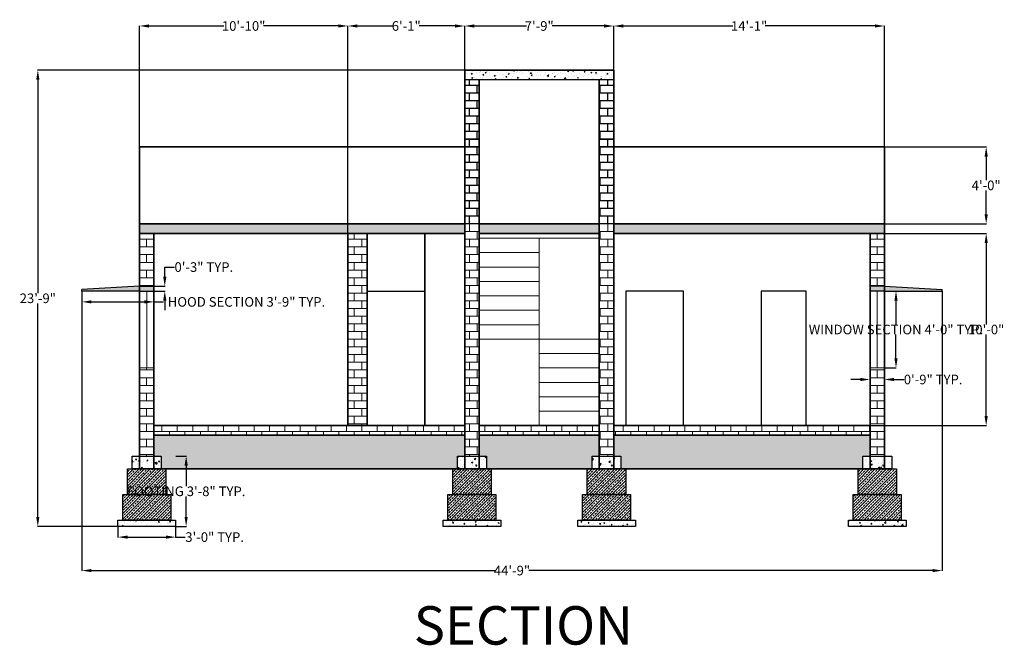
# Model space of a CAD drawing. Units: inches. Extents: x 1966 to 4198, y 2607 to 3884.
# Tile 3 of 8: x 2806 to 3420, y 2607 to 2998. Entities that reach past the tile are written whole.
import ezdxf

# ---------------------------------------------------------------- set-up
doc = ezdxf.new("R2010")
doc.units = ezdxf.units.IN
doc.header["$MEASUREMENT"] = 0
for name, color, linetype, lineweight in [('A-ANNO-TEXT', 4, 'Continuous', 25), ('A-FLOR-STRS', 7, 'Continuous', 18), ('A-GLAZ', 4, 'Continuous', 18), ('A-ROOF', 7, 'Continuous', 25), ('A-SECT', 7, 'Continuous', 35), ('A-SECT-PATT', 8, 'Continuous', 13), ('dimension', 90, 'Continuous', 18), ('door', 17, 'Continuous', 25), ('S-FNDN', 17, 'Continuous', 35)]:
    doc.layers.add(name, color=color, linetype=linetype, lineweight=lineweight)
doc.styles.get("Standard").update_dxf_attribs({"font": 'arial.ttf'})
doc.dimstyles.get("Standard").update_dxf_attribs({"dimtxt": 6, "dimasz": 6, "dimexe": 0.18, "dimexo": 0.0625, "dimgap": 0.09, "dimtad": 0, "dimtih": 1, "dimtoh": 1, "dimdec": 1, "dimzin": 0, "dimdsep": 46, "dimlunit": 3, "dimtxsty": 'Standard', "dimcen": 0.09, "dimadec": 0, "dimazin": 0, "dimtfac": 1, "dimtdec": 1, "dimtofl": 0, "dimtmove": 0, "dimatfit": 3, "dimfxl": 1, "dimtolj": 1, "dimtzin": 0, "dimarcsym": 0})
pattern_1 = [(50, (0, 0), (7.172602, -0.627521), [0.75, -8.25]), (355, (0, 0), (-1.387513, 7.521921), [0.6, -6.6]), (100.45144, (0.598, -0.052), (5.785088, 6.8944), [0.637402, -7.011421]), (46.1842, (0, 2), (10.672413, -1.655193), [1.125, -12.375]), (96.63564, (0.889, 1.862), (9.34662, 9.741186), [0.956103, -10.517138]), (351.18416, (0, 2), (9.34662, 9.741186), [0.9, -9.9]), (21, (1, 1.5), (5.9690705, -4.026189), [0.75, -8.25]), (326, (1, 1.5), (2.433153, 7.2515), [0.6, -6.6]), (71.45144, (1.4974, 1.1645), (8.402224, 3.225312), [0.637402, -7.011421]), (37.5, (0, 0), (0.1215986, 3.3289385), [0, -6.52, 0, -6.7, 0, -6.625]), (7.5, (0, 0), (2.6306954, 3.944117), [0, -3.82, 0, -6.37, 0, -2.525]), (327.5, (-2.23, 0), (5.3382244, -0.2255487), [0, -2.5, 0, -7.8, 0, -10.35]), (317.5, (-3.23, 0), (5.8318617, 1.00105), [0, -3.25, 0, -5.18, 0, -7.35])]

# ---------------------------------------------------------------- blocks, each defined once
blk = doc.blocks.new('FOUNDATION')
at = {"layer": 'door', "transparency": 33554577}
h = blk.add_hatch(dxfattribs=at)
h.set_pattern_fill('AR-CONC', color=256)
h.set_pattern_definition(pattern_1)
h.paths.add_polyline_path([(2817.43, 2606.1), (2817.43, 2602.1), (2853.43, 2602.1), (2853.43, 2606.1)])
h.paths.add_polyline_path([(2844.43, 2638.1), (2844.43, 2646.1), (2826.43, 2646.1), (2826.43, 2638.1)])
h = blk.add_hatch(dxfattribs=at)
h.set_pattern_fill('ANSI33', color=256, scale=10)
h.paths.add_polyline_path([(2847.43, 2622.1), (2847.43, 2638.1), (2823.43, 2638.1), (2823.43, 2622.1)])
h.paths.add_polyline_path([(2850.43, 2606.1), (2850.43, 2622.1), (2820.43, 2622.1), (2820.43, 2606.1)])
at = {"layer": 'door'}
for p, q in [((2826.43, 2646.1), (2844.43, 2646.1)), ((2826.43, 2638.1), (2826.43, 2646.1)), ((2844.43, 2646.1), (2844.43, 2638.1)), ((2823.43, 2638.1), (2847.43, 2638.1)), ((2823.43, 2622.1), (2823.43, 2638.1)), ((2844.43, 2638.1), (2826.43, 2638.1)), ((2847.43, 2638.1), (2847.43, 2622.1)), ((2820.43, 2622.1), (2850.43, 2622.1)), ((2820.43, 2606.1), (2820.43, 2622.1)), ((2847.43, 2622.1), (2823.43, 2622.1)), ((2850.43, 2622.1), (2850.43, 2606.1)), ((2817.43, 2606.1), (2853.43, 2606.1)), ((2817.43, 2602.1), (2817.43, 2606.1)), ((2850.43, 2606.1), (2820.43, 2606.1)), ((2853.43, 2606.1), (2853.43, 2602.1)), ((2853.43, 2602.1), (2817.43, 2602.1))]:
    blk.add_line(p, q, dxfattribs=at)
blk = doc.blocks.new('WINDOW-SECTION')
blk.add_line((4.5, 0), (4.5, 48))
blk.add_lwpolyline([(0, 48), (9, 48), (9, 0), (0, 0)], close=True)
blk = doc.blocks.new('WINDOW-HOOD-SECTION')
for p, q in [((36, 3), (0, 1)), ((0, 0), (0, 1)), ((36, 0), (0, 0)), ((36, 3), (45, 3)), ((36, 0), (45, 0))]:
    blk.add_line(p, q)
blk = doc.blocks.new('*D45')
at = {"layer": 'Defpoints', "color": 0, "transparency": 16777216}
for p in [(2902.94, 2725.47), (2909.54, 2725.47), (2902.94, 2681.47)]:
    blk.add_point(p, dxfattribs=at)
at = {"layer": 'dimension', "color": 0, "lineweight": -2, "transparency": 16777216}
for p, q in [((2903, 2725.47), (2909.72, 2725.47)), ((2909.54, 2719.47), (2909.54, 2706.66)), ((2909.54, 2687.47), (2909.54, 2700.27)), ((2903, 2681.47), (2909.72, 2681.47))]:
    blk.add_line(p, q, dxfattribs=at)
at = {"layer": 'dimension', "color": 0, "transparency": 16777216}
for points in [[(2908.54, 2719.47), (2910.54, 2719.47), (2909.54, 2725.47)], [(2908.54, 2687.47), (2910.54, 2687.47), (2909.54, 2681.47)]]:
    blk.add_solid(points, dxfattribs=at)
at = {"layer": 'dimension', "color": 0, "transparency": 16777216, "insert": (2909.54, 2703.47), "char_height": 6, "attachment_point": 5}
blk.add_mtext('\\A1;FOOTING 3\'-8" TYP.', dxfattribs=at)
blk = doc.blocks.new('*D46')
at = {"layer": 'Defpoints', "color": 0, "transparency": 16777216}
for p in [(2866.94, 2681.47), (2902.94, 2681.47), (2902.94, 2674.87)]:
    blk.add_point(p, dxfattribs=at)
at = {"layer": 'dimension', "color": 0, "lineweight": -2, "transparency": 16777216}
for p, q in [((2866.94, 2681.4), (2866.94, 2674.69)), ((2902.94, 2681.4), (2902.94, 2674.69)), ((2872.94, 2674.87), (2896.94, 2674.87)), ((2902.94, 2674.87), (2908.94, 2674.87))]:
    blk.add_line(p, q, dxfattribs=at)
at = {"layer": 'dimension', "color": 0, "transparency": 16777216}
for points in [[(2872.94, 2675.87), (2872.94, 2673.87), (2866.94, 2674.87)], [(2896.94, 2675.87), (2896.94, 2673.87), (2902.94, 2674.87)]]:
    blk.add_solid(points, dxfattribs=at)
at = {"layer": 'dimension', "color": 0, "transparency": 16777216, "insert": (2927.32, 2674.87), "char_height": 6, "attachment_point": 5}
blk.add_mtext('\\A1;3\'-0" TYP.', dxfattribs=at)
blk = doc.blocks.new('*D71')
at = {"layer": 'Defpoints', "color": 0, "transparency": 16777216}
for p in [(2844.44, 2828.47), (2889.44, 2828.47), (2889.44, 2821.72)]:
    blk.add_point(p, dxfattribs=at)
at = {"layer": 'dimension', "color": 0, "lineweight": -2, "transparency": 16777216}
for p, q in [((2844.44, 2828.4), (2844.44, 2821.54)), ((2889.44, 2828.4), (2889.44, 2821.54)), ((2850.44, 2821.72), (2883.44, 2821.72)), ((2889.44, 2821.72), (2895.44, 2821.72))]:
    blk.add_line(p, q, dxfattribs=at)
at = {"layer": 'dimension', "color": 0, "transparency": 16777216}
for points in [[(2850.44, 2822.72), (2850.44, 2820.72), (2844.44, 2821.72)], [(2883.44, 2822.72), (2883.44, 2820.72), (2889.44, 2821.72)]]:
    blk.add_solid(points, dxfattribs=at)
at = {"layer": 'dimension', "color": 0, "transparency": 16777216, "insert": (2947.19, 2821.72), "char_height": 6, "attachment_point": 5}
blk.add_mtext('\\A1;HOOD SECTION 3\'-9" TYP.', dxfattribs=at)
blk = doc.blocks.new('*D72')
at = {"layer": 'Defpoints', "color": 0, "transparency": 16777216}
for p in [(2889.44, 2831.47), (2889.44, 2828.47), (2896.19, 2831.47)]:
    blk.add_point(p, dxfattribs=at)
at = {"layer": 'dimension', "color": 0, "lineweight": -2, "transparency": 16777216}
for p, q in [((2896.19, 2837.47), (2896.19, 2843.47)), ((2896.19, 2843.47), (2902.19, 2843.47)), ((2889.5, 2831.47), (2896.37, 2831.47)), ((2889.5, 2828.47), (2896.37, 2828.47)), ((2896.19, 2822.47), (2896.19, 2816.47))]:
    blk.add_line(p, q, dxfattribs=at)
at = {"layer": 'dimension', "color": 0, "transparency": 16777216}
for points in [[(2895.19, 2837.47), (2897.19, 2837.47), (2896.19, 2831.47)], [(2895.19, 2822.47), (2897.19, 2822.47), (2896.19, 2828.47)]]:
    blk.add_solid(points, dxfattribs=at)
at = {"layer": 'dimension', "color": 0, "transparency": 16777216, "insert": (2920.57, 2843.47), "char_height": 6, "attachment_point": 5}
blk.add_mtext('\\A1;0\'-3" TYP.', dxfattribs=at)
blk = doc.blocks.new('*D73')
at = {"layer": 'Defpoints', "color": 0, "transparency": 16777216}
for p in [(3345.44, 2828.47), (3352.64, 2828.47), (3345.44, 2780.47)]:
    blk.add_point(p, dxfattribs=at)
at = {"layer": 'dimension', "color": 0, "lineweight": -2, "transparency": 16777216}
for p, q in [((3345.5, 2828.47), (3352.82, 2828.47)), ((3352.64, 2822.47), (3352.64, 2807.66)), ((3352.64, 2786.47), (3352.64, 2801.27)), ((3345.5, 2780.47), (3352.82, 2780.47))]:
    blk.add_line(p, q, dxfattribs=at)
at = {"layer": 'dimension', "color": 0, "transparency": 16777216}
for points in [[(3351.64, 2822.47), (3353.64, 2822.47), (3352.64, 2828.47)], [(3351.64, 2786.47), (3353.64, 2786.47), (3352.64, 2780.47)]]:
    blk.add_solid(points, dxfattribs=at)
at = {"layer": 'dimension', "color": 0, "transparency": 16777216, "insert": (3352.64, 2804.47), "char_height": 6, "attachment_point": 5}
blk.add_mtext('\\A1;WINDOW SECTION 4\'-0" TYP.', dxfattribs=at)
blk = doc.blocks.new('*D74')
at = {"layer": 'Defpoints', "color": 0, "transparency": 16777216}
for p in [(3336.44, 2780.47), (3345.44, 2780.47), (3345.44, 2773.27)]:
    blk.add_point(p, dxfattribs=at)
at = {"layer": 'dimension', "color": 0, "lineweight": -2, "transparency": 16777216}
for p, q in [((3336.44, 2780.4), (3336.44, 2773.09)), ((3345.44, 2780.4), (3345.44, 2773.09)), ((3330.44, 2773.27), (3324.44, 2773.27)), ((3351.44, 2773.27), (3357.44, 2773.27))]:
    blk.add_line(p, q, dxfattribs=at)
at = {"layer": 'dimension', "color": 0, "transparency": 16777216}
for points in [[(3330.44, 2774.27), (3330.44, 2772.27), (3336.44, 2773.27)], [(3351.44, 2774.27), (3351.44, 2772.27), (3345.44, 2773.27)]]:
    blk.add_solid(points, dxfattribs=at)
at = {"layer": 'dimension', "color": 0, "transparency": 16777216, "insert": (3375.82, 2773.27), "char_height": 6, "attachment_point": 5}
blk.add_mtext('\\A1;0\'-9" TYP.', dxfattribs=at)
blk = doc.blocks.new('*D112')
at = {"layer": 'Defpoints', "color": 0, "transparency": 16777216}
for p in [(2844.44, 2828.47), (3381.44, 2828.47), (3381.44, 2653.97)]:
    blk.add_point(p, dxfattribs=at)
at = {"layer": 'dimension', "color": 0, "lineweight": -2, "transparency": 16777216}
for p, q in [((2844.44, 2828.4), (2844.44, 2653.79)), ((3381.44, 2828.4), (3381.44, 2653.79)), ((2850.44, 2653.97), (3102.42, 2653.97)), ((3375.44, 2653.97), (3123.46, 2653.97))]:
    blk.add_line(p, q, dxfattribs=at)
at = {"layer": 'dimension', "color": 0, "transparency": 16777216}
for points in [[(2850.44, 2654.97), (2850.44, 2652.97), (2844.44, 2653.97)], [(3375.44, 2654.97), (3375.44, 2652.97), (3381.44, 2653.97)]]:
    blk.add_solid(points, dxfattribs=at)
at = {"layer": 'dimension', "color": 0, "transparency": 16777216, "insert": (3112.94, 2653.97), "char_height": 6, "attachment_point": 5}
blk.add_mtext('\\A1;44\'-9"', dxfattribs=at)
blk = doc.blocks.new('*D113')
at = {"layer": 'Defpoints', "color": 0, "transparency": 16777216}
for p in [(2816.94, 2966.47), (3083.44, 2966.47), (2866.94, 2681.47)]:
    blk.add_point(p, dxfattribs=at)
at = {"layer": 'dimension', "color": 0, "lineweight": -2, "transparency": 16777216}
for p, q in [((3083.38, 2966.47), (2816.76, 2966.47)), ((2816.94, 2960.47), (2816.94, 2827.12)), ((2816.94, 2687.47), (2816.94, 2820.81)), ((2866.88, 2681.47), (2816.76, 2681.47))]:
    blk.add_line(p, q, dxfattribs=at)
at = {"layer": 'dimension', "color": 0, "transparency": 16777216}
for points in [[(2815.94, 2960.47), (2817.94, 2960.47), (2816.94, 2966.47)], [(2815.94, 2687.47), (2817.94, 2687.47), (2816.94, 2681.47)]]:
    blk.add_solid(points, dxfattribs=at)
at = {"layer": 'dimension', "color": 0, "transparency": 16777216, "insert": (2816.94, 2823.97), "char_height": 6, "attachment_point": 5}
blk.add_mtext('\\A1;23\'-9"', dxfattribs=at)
blk = doc.blocks.new('*D114')
at = {"layer": 'Defpoints', "color": 0, "transparency": 16777216}
for p in [(3336.44, 2864.47), (3408.94, 2864.47), (3336.44, 2744.47)]:
    blk.add_point(p, dxfattribs=at)
at = {"layer": 'dimension', "color": 0, "lineweight": -2, "transparency": 16777216}
for p, q in [((3336.5, 2864.47), (3409.12, 2864.47)), ((3408.94, 2858.47), (3408.94, 2807.62)), ((3408.94, 2750.47), (3408.94, 2801.31)), ((3336.5, 2744.47), (3409.12, 2744.47))]:
    blk.add_line(p, q, dxfattribs=at)
at = {"layer": 'dimension', "color": 0, "transparency": 16777216}
for points in [[(3407.94, 2858.47), (3409.94, 2858.47), (3408.94, 2864.47)], [(3407.94, 2750.47), (3409.94, 2750.47), (3408.94, 2744.47)]]:
    blk.add_solid(points, dxfattribs=at)
at = {"layer": 'dimension', "color": 0, "transparency": 16777216, "insert": (3408.94, 2804.47), "char_height": 6, "attachment_point": 5}
blk.add_mtext('\\A1;10\'-0"', dxfattribs=at)
blk = doc.blocks.new('*D115')
at = {"layer": 'Defpoints', "color": 0, "transparency": 16777216}
for p in [(3010.44, 2993.97), (2880.44, 2864.47), (3010.44, 2864.47)]:
    blk.add_point(p, dxfattribs=at)
at = {"layer": 'dimension', "color": 0, "lineweight": -2, "transparency": 16777216}
for p, q in [((2880.44, 2864.53), (2880.44, 2994.15)), ((2886.44, 2993.97), (2933, 2993.97)), ((3004.44, 2993.97), (2957.88, 2993.97)), ((3010.44, 2864.53), (3010.44, 2994.15))]:
    blk.add_line(p, q, dxfattribs=at)
at = {"layer": 'dimension', "color": 0, "transparency": 16777216}
for points in [[(2886.44, 2994.97), (2886.44, 2992.97), (2880.44, 2993.97)], [(3004.44, 2994.97), (3004.44, 2992.97), (3010.44, 2993.97)]]:
    blk.add_solid(points, dxfattribs=at)
at = {"layer": 'dimension', "color": 0, "transparency": 16777216, "insert": (2945.44, 2993.97), "char_height": 6, "attachment_point": 5}
blk.add_mtext('\\A1;10\'-10"', dxfattribs=at)
blk = doc.blocks.new('*D116')
at = {"layer": 'Defpoints', "color": 0, "transparency": 16777216}
for p in [(3083.44, 2993.97), (3083.44, 2918.47), (3010.44, 2864.47)]:
    blk.add_point(p, dxfattribs=at)
at = {"layer": 'dimension', "color": 0, "lineweight": -2, "transparency": 16777216}
for p, q in [((3010.44, 2864.53), (3010.44, 2994.15)), ((3016.44, 2993.97), (3038.86, 2993.97)), ((3077.44, 2993.97), (3055.02, 2993.97)), ((3083.44, 2918.53), (3083.44, 2994.15))]:
    blk.add_line(p, q, dxfattribs=at)
at = {"layer": 'dimension', "color": 0, "transparency": 16777216}
for points in [[(3016.44, 2994.97), (3016.44, 2992.97), (3010.44, 2993.97)], [(3077.44, 2994.97), (3077.44, 2992.97), (3083.44, 2993.97)]]:
    blk.add_solid(points, dxfattribs=at)
at = {"layer": 'dimension', "color": 0, "transparency": 16777216, "insert": (3046.94, 2993.97), "char_height": 6, "attachment_point": 5}
blk.add_mtext('\\A1;6\'-1"', dxfattribs=at)
blk = doc.blocks.new('*D117')
at = {"layer": 'Defpoints', "color": 0, "transparency": 16777216}
for p in [(3176.44, 2993.97), (3083.44, 2966.47), (3176.44, 2966.42)]:
    blk.add_point(p, dxfattribs=at)
at = {"layer": 'dimension', "color": 0, "lineweight": -2, "transparency": 16777216}
for p, q in [((3083.44, 2966.53), (3083.44, 2994.15)), ((3089.44, 2993.97), (3121.9, 2993.97)), ((3170.44, 2993.97), (3137.98, 2993.97)), ((3176.44, 2966.49), (3176.44, 2994.15))]:
    blk.add_line(p, q, dxfattribs=at)
at = {"layer": 'dimension', "color": 0, "transparency": 16777216}
for points in [[(3089.44, 2994.97), (3089.44, 2992.97), (3083.44, 2993.97)], [(3170.44, 2994.97), (3170.44, 2992.97), (3176.44, 2993.97)]]:
    blk.add_solid(points, dxfattribs=at)
at = {"layer": 'dimension', "color": 0, "transparency": 16777216, "insert": (3129.94, 2993.97), "char_height": 6, "attachment_point": 5}
blk.add_mtext('\\A1;7\'-9"', dxfattribs=at)
blk = doc.blocks.new('*D118')
at = {"layer": 'Defpoints', "color": 0, "transparency": 16777216}
for p in [(3345.44, 2993.97), (3176.44, 2918.47), (3345.44, 2918.47)]:
    blk.add_point(p, dxfattribs=at)
at = {"layer": 'dimension', "color": 0, "lineweight": -2, "transparency": 16777216}
for p, q in [((3176.44, 2918.53), (3176.44, 2994.15)), ((3182.44, 2993.97), (3250.83, 2993.97)), ((3339.44, 2993.97), (3271.05, 2993.97)), ((3345.44, 2918.53), (3345.44, 2994.15))]:
    blk.add_line(p, q, dxfattribs=at)
at = {"layer": 'dimension', "color": 0, "transparency": 16777216}
for points in [[(3182.44, 2994.97), (3182.44, 2992.97), (3176.44, 2993.97)], [(3339.44, 2994.97), (3339.44, 2992.97), (3345.44, 2993.97)]]:
    blk.add_solid(points, dxfattribs=at)
at = {"layer": 'dimension', "color": 0, "transparency": 16777216, "insert": (3260.94, 2993.97), "char_height": 6, "attachment_point": 5}
blk.add_mtext('\\A1;14\'-1"', dxfattribs=at)
blk = doc.blocks.new('*D119')
at = {"layer": 'Defpoints', "color": 0, "transparency": 16777216}
for p in [(3345.44, 2918.47), (3408.94, 2918.47), (3345.44, 2870.47)]:
    blk.add_point(p, dxfattribs=at)
at = {"layer": 'dimension', "color": 0, "lineweight": -2, "transparency": 16777216}
for p, q in [((3345.5, 2918.47), (3409.12, 2918.47)), ((3408.94, 2912.47), (3408.94, 2897.62)), ((3408.94, 2876.47), (3408.94, 2891.31)), ((3345.5, 2870.47), (3409.12, 2870.47))]:
    blk.add_line(p, q, dxfattribs=at)
at = {"layer": 'dimension', "color": 0, "transparency": 16777216}
for points in [[(3407.94, 2912.47), (3409.94, 2912.47), (3408.94, 2918.47)], [(3407.94, 2876.47), (3409.94, 2876.47), (3408.94, 2870.47)]]:
    blk.add_solid(points, dxfattribs=at)
at = {"layer": 'dimension', "color": 0, "transparency": 16777216, "insert": (3408.94, 2894.47), "char_height": 6, "attachment_point": 5}
blk.add_mtext('\\A1;4\'-0"', dxfattribs=at)

msp = doc.modelspace()

# ---------------------------------------------------------------- hatches: boundary and pattern name
at = {"layer": 'A-SECT-PATT', "transparency": 33554577}
h = msp.add_hatch(dxfattribs=at)
h.set_pattern_fill('AR-CONC', color=256)
h.set_pattern_definition(pattern_1)
h.paths.add_polyline_path([(3176.44, 2966.42), (3083.44, 2966.47), (3083.44, 2960.47), (3176.44, 2960.42)])
h = msp.add_hatch(dxfattribs=at)
h.set_pattern_fill('AR-B816C', color=256, scale=0.6)
h.paths.add_polyline_path([(3092.44, 2960.46), (3083.44, 2960.47), (3083.44, 2870.47), (3092.44, 2870.47)])
h.paths.add_polyline_path([(3176.44, 2960.42), (3167.44, 2960.43), (3167.44, 2870.47), (3176.44, 2870.47)])
h = msp.add_hatch(dxfattribs=at)
h.set_pattern_fill('AR-B816', color=256, scale=0.6)
h.paths.add_polyline_path([(2889.44, 2780.47), (2880.44, 2780.47), (2880.44, 2725.47), (2889.44, 2725.47)])
h.paths.add_polyline_path([(2889.44, 2864.47), (2880.44, 2864.47), (2880.44, 2831.47), (2889.44, 2831.47)])
h.paths.add_polyline_path([(3022.44, 2864.47), (3010.44, 2864.47), (3010.44, 2744.47), (3022.44, 2744.47)])
h.paths.add_polyline_path([(3092.44, 2870.44), (3083.44, 2870.44), (3083.44, 2725.47), (3092.44, 2725.47)])
h.paths.add_polyline_path([(3176.44, 2870.73), (3167.44, 2870.73), (3167.44, 2725.47), (3176.44, 2725.47)])
h.paths.add_polyline_path([(3345.44, 2864.47), (3336.44, 2864.47), (3336.44, 2831.47), (3345.44, 2831.47)])
h.paths.add_polyline_path([(3345.44, 2780.47), (3336.44, 2780.47), (3336.44, 2725.47), (3345.44, 2725.47)])
h.paths.add_polyline_path([(3083.44, 2744.47), (3058.44, 2744.47), (2889.44, 2744.47), (2889.44, 2738.47), (3083.44, 2738.47)])
h.paths.add_polyline_path([(3129.94, 2744.47), (3092.44, 2744.47), (3092.44, 2738.47), (3129.94, 2738.47)])
h.paths.add_polyline_path([(3167.44, 2744.47), (3129.94, 2744.47), (3129.94, 2738.47), (3167.44, 2738.47)])
h.paths.add_polyline_path([(3336.44, 2744.47), (3176.44, 2744.47), (3176.44, 2738.47), (3336.44, 2738.47)])
h = msp.add_hatch(dxfattribs=at)
h.set_pattern_fill('AR-CONC', color=256)
h.set_pattern_definition(pattern_1)
h.paths.add_polyline_path([(3083.44, 2864.47), (3083.44, 2870.47), (2880.44, 2870.47), (2880.44, 2864.47)])
h.paths.add_polyline_path([(3167.44, 2864.47), (3167.44, 2870.47), (3092.44, 2870.47), (3092.44, 2864.47)])
h.paths.add_polyline_path([(3176.44, 2870.47), (3176.44, 2864.47), (3345.44, 2864.47), (3345.44, 2870.47)])
h = msp.add_hatch(dxfattribs=at)
h.set_pattern_fill('AR-CONC', color=256)
h.set_pattern_definition(pattern_1)
h.paths.add_polyline_path([(2880.44, 2831.47), (2844.44, 2829.47), (2844.44, 2828.47), (2880.44, 2828.47)])
h.paths.add_polyline_path([(2889.44, 2831.47), (2880.44, 2831.47), (2880.44, 2828.47), (2889.44, 2828.47)])
h.paths.add_polyline_path([(3345.44, 2831.47), (3336.44, 2831.47), (3336.44, 2828.47), (3345.44, 2828.47)])
h.paths.add_polyline_path([(3345.44, 2831.47), (3345.44, 2828.47), (3381.44, 2828.47), (3381.44, 2829.47)])
h = msp.add_hatch(dxfattribs=at)
h.set_pattern_fill('AR-CONC', color=256)
h.set_pattern_definition(pattern_1)
h.paths.add_polyline_path([(3078.94, 2725.47), (3083.44, 2725.47), (3083.44, 2738.47), (2889.44, 2738.47), (2889.44, 2725.47), (2893.94, 2725.47), (2893.94, 2717.47), (2896.94, 2717.47), (3078.94, 2717.47)])
h.paths.add_polyline_path([(3167.44, 2738.47), (3092.44, 2738.47), (3092.44, 2725.47), (3096.94, 2725.47), (3096.94, 2717.47), (3099.94, 2717.47), (3162.94, 2717.47), (3162.94, 2725.47), (3167.44, 2725.47)])
h.paths.add_polyline_path([(3336.44, 2738.47), (3176.44, 2738.47), (3176.44, 2725.47), (3180.94, 2725.47), (3180.94, 2717.47), (3183.94, 2717.47), (3331.94, 2717.47), (3331.94, 2725.47), (3336.44, 2725.47)])

# ---------------------------------------------------------------- linework, layer by layer
at = {"layer": 'A-FLOR-STRS'}
for p, q in [((3092.44, 2861.47), (3167.44, 2861.47)), ((3129.94, 2744.47), (3129.94, 2861.47)), ((3092.44, 2852.47), (3129.94, 2852.47)), ((3092.44, 2843.47), (3129.94, 2843.47)), ((3092.44, 2834.47), (3129.94, 2834.47)), ((3092.44, 2825.47), (3129.94, 2825.47)), ((3092.44, 2816.47), (3129.94, 2816.47)), ((3092.44, 2807.47), (3129.94, 2807.47)), ((3092.44, 2798.47), (3167.44, 2798.47)), ((3129.94, 2789.47), (3167.44, 2789.47)), ((3129.94, 2780.47), (3167.44, 2780.47)), ((3129.94, 2771.47), (3167.44, 2771.47)), ((3129.94, 2762.47), (3167.44, 2762.47)), ((3129.94, 2753.47), (3167.44, 2753.47))]:
    msp.add_line(p, q, dxfattribs=at)
at = {"layer": 'A-SECT'}
for p, q in [((3083.44, 2966.47), (3176.44, 2966.42)), ((3083.44, 2966.47), (3083.44, 2960.47)), ((3176.44, 2966.42), (3176.44, 2960.42)), ((3083.44, 2864.47), (3083.44, 2960.47)), ((3083.44, 2960.47), (3176.44, 2960.42)), ((3092.44, 2864.47), (3092.44, 2960.47)), ((3167.44, 2960.42), (3167.44, 2864.47)), ((3176.44, 2960.42), (3176.44, 2864.47)), ((2880.44, 2918.47), (2880.44, 2717.47)), ((2880.44, 2918.47), (3083.44, 2918.47)), ((3176.44, 2918.47), (3345.44, 2918.47)), ((3345.44, 2918.47), (3345.44, 2717.47)), ((2880.44, 2870.47), (3083.44, 2870.47)), ((3092.44, 2870.47), (3167.44, 2870.47)), ((3176.44, 2870.47), (3345.44, 2870.47)), ((2880.44, 2864.47), (3083.44, 2864.47)), ((2889.44, 2864.47), (2889.44, 2717.47)), ((3010.44, 2864.47), (3010.44, 2744.47)), ((3022.44, 2744.47), (3022.44, 2864.47)), ((3058.44, 2744.47), (3058.44, 2864.47)), ((3083.44, 2864.47), (3083.44, 2717.47)), ((3092.44, 2864.47), (3092.44, 2717.47)), ((3092.44, 2864.47), (3167.44, 2864.47)), ((3167.44, 2864.47), (3167.44, 2717.47)), ((3176.44, 2864.47), (3176.44, 2717.47)), ((3176.44, 2864.47), (3345.44, 2864.47)), ((3336.44, 2864.47), (3336.44, 2717.47)), ((2889.44, 2744.47), (3083.44, 2744.47)), ((3092.44, 2744.47), (3167.44, 2744.47)), ((3176.44, 2744.47), (3336.44, 2744.47)), ((2889.44, 2738.47), (3083.44, 2738.47)), ((3092.44, 2738.47), (3167.44, 2738.47)), ((3176.44, 2738.47), (3336.44, 2738.47)), ((2880.44, 2717.47), (3345.44, 2717.47))]:
    msp.add_line(p, q, dxfattribs=at)
at = {"layer": 'door'}
for points in [[(3022.44, 2828.47), (3058.44, 2828.47), (3058.44, 2744.47), (3022.44, 2744.47)], [(3183.92, 2744.47), (3219.92, 2744.47), (3219.92, 2828.47), (3183.92, 2828.47)], [(3268.55, 2744.47), (3296.55, 2744.47), (3296.55, 2828.47), (3268.55, 2828.47)]]:
    msp.add_lwpolyline(points, close=True, dxfattribs=at)
at = {"layer": 'S-FNDN'}
for p, q in [((2880.44, 2717.47), (2889.44, 2717.47)), ((3083.44, 2717.47), (3092.44, 2717.47)), ((3167.44, 2717.47), (3176.44, 2717.47)), ((3336.44, 2717.47), (3345.44, 2717.47))]:
    msp.add_line(p, q, dxfattribs=at)

# ---------------------------------------------------------------- block references
at = {"layer": 'A-GLAZ'}
for p in [(2880.44, 2780.47), (3336.44, 2780.47)]:
    msp.add_blockref('WINDOW-SECTION', p, dxfattribs=at)
at = {"layer": 'A-ROOF'}
msp.add_blockref('WINDOW-HOOD-SECTION', (2844.44, 2828.47), dxfattribs=at)
at = {"layer": 'A-ROOF', "extrusion": (0, 0, -1), "zscale": -1}
msp.add_blockref('WINDOW-HOOD-SECTION', (-3381.44, 2828.47), dxfattribs=at)
at = {"layer": 'S-FNDN'}
for p in [(49.51, 79.37), (252.51, 79.37), (336.51, 79.37), (505.51, 79.37)]:
    msp.add_blockref('FOUNDATION', p, dxfattribs=at)

# ---------------------------------------------------------------- texts
at = {"layer": 'A-ANNO-TEXT', "insert": (3120.06, 2631.74), "char_height": 24, "attachment_point": 2}
msp.add_mtext_dynamic_manual_height_columns('SECTION', width=89.9452, gutter_width=1, heights=[0], dxfattribs=at)

# ---------------------------------------------------------------- dimensions: what is measured, and where the dimension line sits
at = {"layer": 'dimension'}
for base, p1, p2, picture, middle in [((3010.44, 2993.97), (2880.44, 2864.47), (3010.44, 2864.47), '*D115', (2945.44, 2993.97)), ((3083.44, 2993.97), (3010.44, 2864.47), (3083.44, 2918.47), '*D116', (3046.94, 2993.97)), ((3176.44, 2993.97), (3083.44, 2966.47), (3176.44, 2966.42), '*D117', (3129.94, 2993.97)), ((3345.44, 2993.97), (3176.44, 2918.47), (3345.44, 2918.47), '*D118', (3260.94, 2993.97)), ((3381.44, 2653.97), (2844.44, 2828.47), (3381.44, 2828.47), '*D112', (3112.94, 2653.97))]:
    dim = msp.add_linear_dim(base=base, p1=p1, p2=p2, dimstyle='Standard', override={"dimdec": 1, "dimlfac": 1, "dimrnd": 0, "dimzin": 1, "dimdsep": 46, "dimlunit": 4, "dimfrac": 2}, dxfattribs=at)
    dim.commit()
    dim.dimension.update_dxf_attribs({"geometry": picture, "text_midpoint": middle})
for base, p1, p2, picture, middle in [((2816.94, 2966.47), (2866.94, 2681.47), (3083.44, 2966.47), '*D113', (2816.94, 2823.97)), ((3408.94, 2918.47), (3345.44, 2870.47), (3345.44, 2918.47), '*D119', (3408.94, 2894.47)), ((3408.94, 2864.47), (3336.44, 2744.47), (3336.44, 2864.47), '*D114', (3408.94, 2804.47))]:
    dim = msp.add_linear_dim(base=base, p1=p1, p2=p2, angle=90, dimstyle='Standard', override={"dimdec": 1, "dimlfac": 1, "dimrnd": 0, "dimzin": 1, "dimdsep": 46, "dimlunit": 4, "dimfrac": 2}, dxfattribs=at)
    dim.commit()
    dim.dimension.update_dxf_attribs({"geometry": picture, "text_midpoint": middle})
for base, p1, p2, text, picture, middle in [((2896.19, 2831.47), (2889.44, 2828.47), (2889.44, 2831.47), '<> TYP.', '*D72', (2920.57, 2843.47)), ((3352.64, 2828.47), (3345.44, 2780.47), (3345.44, 2828.47), 'WINDOW SECTION <> TYP.', '*D73', (3352.64, 2804.47)), ((2909.54, 2725.47), (2902.94, 2681.47), (2902.94, 2725.47), 'FOOTING <> TYP.', '*D45', (2909.54, 2703.47))]:
    dim = msp.add_linear_dim(base=base, p1=p1, p2=p2, angle=90, text=text, dimstyle='Standard', override={"dimdec": 1, "dimlfac": 1, "dimrnd": 0, "dimzin": 1, "dimdsep": 46, "dimlunit": 4, "dimfrac": 2}, dxfattribs=at)
    dim.commit()
    dim.dimension.update_dxf_attribs({"geometry": picture, "text_midpoint": middle})
for base, p1, p2, text, picture, middle in [((2889.44, 2821.72), (2844.44, 2828.47), (2889.44, 2828.47), 'HOOD SECTION <> TYP.', '*D71', (2947.19, 2821.72)), ((3345.44, 2773.27), (3336.44, 2780.47), (3345.44, 2780.47), '<> TYP.', '*D74', (3375.82, 2773.27)), ((2902.94, 2674.87), (2866.94, 2681.47), (2902.94, 2681.47), '<> TYP.', '*D46', (2927.32, 2674.87))]:
    dim = msp.add_linear_dim(base=base, p1=p1, p2=p2, text=text, dimstyle='Standard', override={"dimdec": 1, "dimlfac": 1, "dimrnd": 0, "dimzin": 1, "dimdsep": 46, "dimlunit": 4, "dimfrac": 2}, dxfattribs=at)
    dim.commit()
    dim.dimension.update_dxf_attribs({"geometry": picture, "text_midpoint": middle})

doc.saveas('drawing.dxf')
